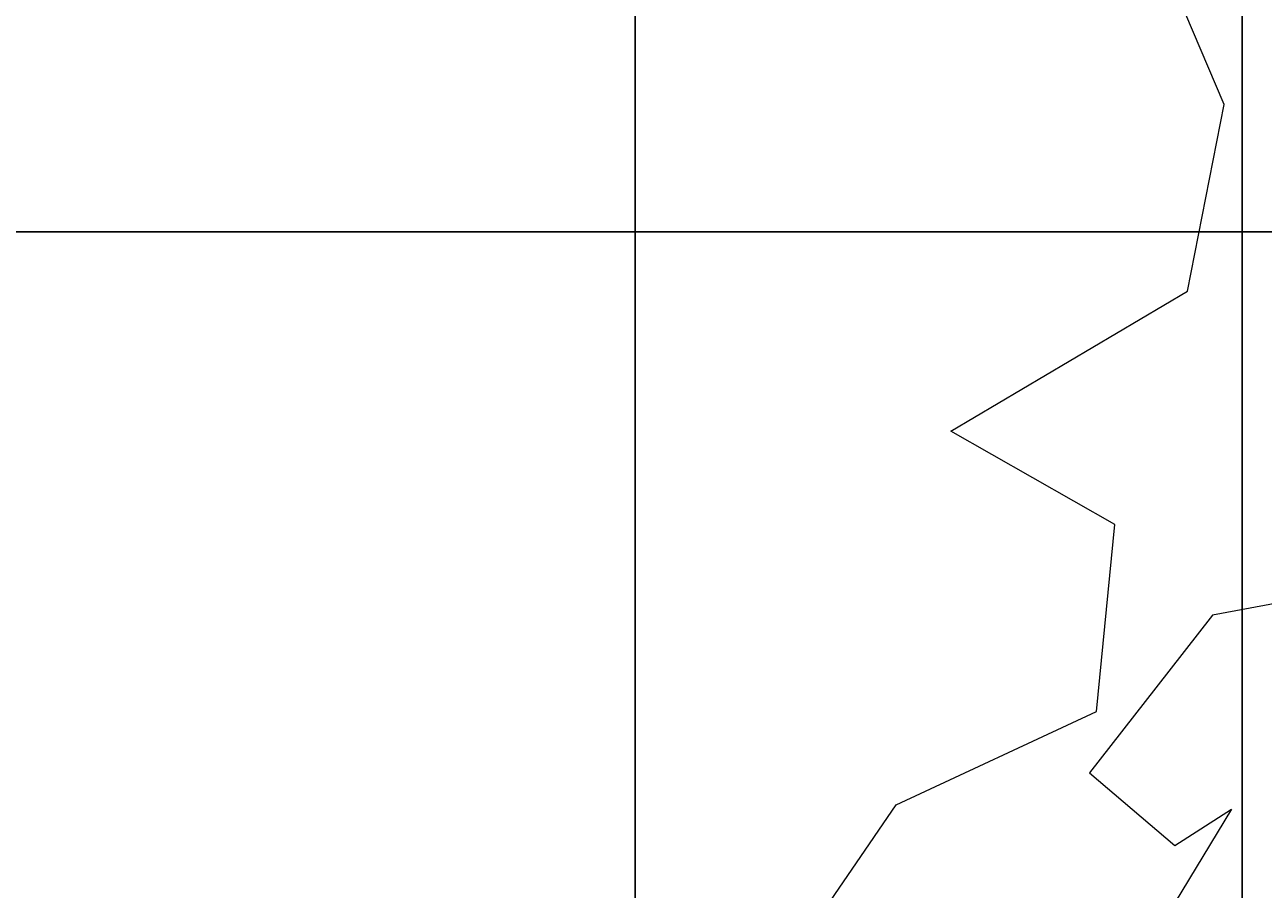
# Model space of a CAD drawing. Units: inches. Extents: x -26 to 776, y -22 to 650.
# Tile 48 of 62: x 506 to 586, y 102 to 158. Entities that reach past the tile are written whole.
import ezdxf

# ---------------------------------------------------------------- set-up
doc = ezdxf.new("R2010")
doc.units = ezdxf.units.IN
doc.header["$MEASUREMENT"] = 0
doc.layers.add('A-ANNO-DIMS', color=2, linetype='Continuous', lineweight=18)
doc.layers.add('L-PLNT-TREE', color=94, linetype='Continuous', lineweight=18)
doc.styles.get("Standard").update_dxf_attribs({"font": 'arial.ttf'})
doc.dimstyles.get("Standard").update_dxf_attribs({"dimtxt": 0.5625, "dimasz": 0.18, "dimexe": 0.18, "dimexo": 0.0625, "dimgap": 0.09, "dimtad": 0, "dimtih": 1, "dimtoh": 1, "dimdec": 4, "dimzin": 0, "dimdsep": 46, "dimlunit": 4, "dimtxsty": 'Standard', "dimcen": 0.09, "dimadec": 0, "dimazin": 0, "dimtfac": 1, "dimtdec": 4, "dimtofl": 0, "dimtmove": 0, "dimatfit": 3, "dimfxl": 1, "dimtolj": 1, "dimtzin": 0, "dimarcsym": 0})

# ---------------------------------------------------------------- blocks, each defined once
blk = doc.blocks.new('Tree - type 3 evergreen elevation')
blk.add_lwpolyline([(-39.2518, 74.099), (-42.2711, 73.5461), (-44.8592, 70.2282), (-47.8786, 66.3574), (-43.9965, 63.0395), (-41.4085, 64.6985), (-44.3346, 59.8898)])
blk = doc.blocks.new('Tree - type 2 deciduous elevation')
blk.add_lwpolyline([(19.675, 39.077), (23.701, 44.975), (30.027, 47.924), (30.602, 53.823), (25.426, 56.772), (32.903, 61.196), (34.053, 67.094), (30.602, 75.205), (34.628, 89.951), (26.576, 103.222)])
blk = doc.blocks.new('*D20')
at = {"layer": 'A-ANNO-DIMS', "color": 0, "lineweight": -2, "transparency": 16777216}
for p, q in [((425.806, 455.472), (775.335, 455.472)), ((775.155, 455.292), (775.155, 235.854)), ((775.155, 15.662), (775.155, 235.1)), ((425.806, 15.482), (775.335, 15.482))]:
    blk.add_line(p, q, dxfattribs=at)
at = {"layer": 'A-ANNO-DIMS', "color": 0, "transparency": 16777216}
for points in [[(775.125, 455.292), (775.185, 455.292), (775.155, 455.472)], [(775.125, 15.662), (775.185, 15.662), (775.155, 15.482)]]:
    blk.add_solid(points, dxfattribs=at)
at = {"layer": 'Defpoints', "color": 0, "transparency": 16777216}
for p in [(425.743, 455.472), (775.155, 455.472), (425.743, 15.482)]:
    blk.add_point(p, dxfattribs=at)
at = {"layer": 'A-ANNO-DIMS', "color": 0, "transparency": 16777216, "insert": (775.155, 235.477), "char_height": 0.5625, "attachment_point": 5}
blk.add_mtext('\\A1;440', dxfattribs=at)
blk = doc.blocks.new('*D30')
at = {"layer": 'A-ANNO-DIMS', "color": 0, "lineweight": -2, "transparency": 16777216}
for p, q in [((280.68, 144.836), (775.335, 144.836)), ((775.155, 144.656), (775.155, 86.007)), ((775.155, 26.604), (775.155, 85.253)), ((280.68, 26.424), (775.335, 26.424))]:
    blk.add_line(p, q, dxfattribs=at)
at = {"layer": 'A-ANNO-DIMS', "color": 0, "transparency": 16777216}
for points in [[(775.125, 144.656), (775.185, 144.656), (775.155, 144.836)], [(775.125, 26.604), (775.185, 26.604), (775.155, 26.424)]]:
    blk.add_solid(points, dxfattribs=at)
at = {"layer": 'Defpoints', "color": 0, "transparency": 16777216}
for p in [(280.617, 144.836), (775.155, 144.836), (280.617, 26.424)]:
    blk.add_point(p, dxfattribs=at)
at = {"layer": 'A-ANNO-DIMS', "color": 0, "transparency": 16777216, "insert": (775.155, 85.63), "char_height": 0.5625, "attachment_point": 5}
blk.add_mtext('\\A1;118.41', dxfattribs=at)
blk = doc.blocks.new('*D45')
at = {"layer": 'A-ANNO-DIMS', "color": 0, "lineweight": -2, "transparency": 16777216}
for p, q in [((507.738, 408.639), (775.335, 408.639)), ((775.155, 408.459), (775.155, 212.438)), ((775.155, 15.662), (775.155, 211.683)), ((585.998, 15.482), (775.335, 15.482))]:
    blk.add_line(p, q, dxfattribs=at)
at = {"layer": 'A-ANNO-DIMS', "color": 0, "transparency": 16777216}
for points in [[(775.125, 408.459), (775.185, 408.459), (775.155, 408.639)], [(775.125, 15.662), (775.185, 15.662), (775.155, 15.482)]]:
    blk.add_solid(points, dxfattribs=at)
at = {"layer": 'Defpoints', "color": 0, "transparency": 16777216}
for p in [(507.676, 408.639), (775.155, 408.639), (585.935, 15.482)]:
    blk.add_point(p, dxfattribs=at)
at = {"layer": 'A-ANNO-DIMS', "color": 0, "transparency": 16777216, "insert": (775.155, 212.061), "char_height": 0.5625, "attachment_point": 5}
blk.add_mtext('\\A1;393.16', dxfattribs=at)
blk = doc.blocks.new('*D47')
at = {"layer": 'A-ANNO-DIMS', "color": 0, "lineweight": -2, "transparency": 16777216}
for p, q in [((584.343, 199.901), (584.343, -21.315)), ((428.648, 180.243), (428.648, -21.315)), ((428.828, -21.135), (505.483, -21.135)), ((584.163, -21.135), (507.508, -21.135))]:
    blk.add_line(p, q, dxfattribs=at)
at = {"layer": 'A-ANNO-DIMS', "color": 0, "transparency": 16777216}
for points in [[(428.828, -21.105), (428.828, -21.165), (428.648, -21.135)], [(584.163, -21.105), (584.163, -21.165), (584.343, -21.135)]]:
    blk.add_solid(points, dxfattribs=at)
at = {"layer": 'Defpoints', "color": 0, "transparency": 16777216}
for p in [(584.343, 199.963), (428.648, 180.305), (584.343, -21.135)]:
    blk.add_point(p, dxfattribs=at)
at = {"layer": 'A-ANNO-DIMS', "color": 0, "transparency": 16777216, "insert": (506.496, -21.135), "char_height": 0.5625, "attachment_point": 5}
blk.add_mtext('\\A1;155.7', dxfattribs=at)
blk = doc.blocks.new('*D48')
at = {"layer": 'A-ANNO-DIMS', "color": 0, "lineweight": -2, "transparency": 16777216}
for p, q in [((545.033, 67.415), (545.033, 649.856)), ((545.213, 649.676), (640.879, 649.676)), ((738.57, 649.676), (642.904, 649.676)), ((738.75, 50.911), (738.75, 649.856))]:
    blk.add_line(p, q, dxfattribs=at)
at = {"layer": 'A-ANNO-DIMS', "color": 0, "transparency": 16777216}
for points in [[(545.213, 649.706), (545.213, 649.646), (545.033, 649.676)], [(738.57, 649.706), (738.57, 649.646), (738.75, 649.676)]]:
    blk.add_solid(points, dxfattribs=at)
at = {"layer": 'Defpoints', "color": 0, "transparency": 16777216}
for p in [(738.75, 649.676), (545.033, 67.352), (738.75, 50.848)]:
    blk.add_point(p, dxfattribs=at)
at = {"layer": 'A-ANNO-DIMS', "color": 0, "transparency": 16777216, "insert": (641.892, 649.676), "char_height": 0.5625, "attachment_point": 5}
blk.add_mtext('\\A1;193.7', dxfattribs=at)

msp = doc.modelspace()

# ---------------------------------------------------------------- block references
at = {"layer": 'L-PLNT-TREE'}
for name, p, xscale, yscale, zscale in [('Tree - type 2 deciduous elevation', (513.3241, 15.4824), 2.050905272406618, 2.050905272406618, 2.050905272406618), ('Tree - type 3 evergreen elevation', (642.5048, 15.4824), 1.421226385586178, 1.421226385586178, 1.421226385586178)]:
    msp.add_blockref(name, p, dxfattribs=dict(at, xscale=xscale, yscale=yscale, zscale=zscale))

# ---------------------------------------------------------------- dimensions: what is measured, and where the dimension line sits
at = {"layer": 'A-ANNO-DIMS'}
for base, p1, p2, picture, middle in [((738.7503, 649.6763), (545.0331, 67.3523), (738.7503, 50.8482), '*D48', (641.8917, 649.6763)), ((584.3428, -21.1349), (428.6484, 180.3054), (584.3428, 199.9634), '*D47', (506.4956, -21.1349))]:
    dim = msp.add_linear_dim(base=base, p1=p1, p2=p2, dimstyle='Standard', override={"dimdec": 1, "dimlfac": 1, "dimrnd": 0, "dimzin": 0, "dimdsep": 46, "dimlunit": 2}, dxfattribs=at)
    dim.commit()
    dim.dimension.update_dxf_attribs({"geometry": picture, "text_midpoint": middle})
for base, p1, p2, override, picture, middle in [((775.1553, 455.4717), (425.7434, 15.4824), (425.7434, 455.4717), {"dimdec": 0, "dimlfac": 1, "dimrnd": 0, "dimzin": 0, "dimdsep": 46, "dimlunit": 2}, '*D20', (775.1553, 235.477)), ((775.1553, 408.6389), (585.9354, 15.4824), (507.6759, 408.6389), {"dimdec": 2, "dimlfac": 1, "dimrnd": 0, "dimzin": 0, "dimdsep": 46, "dimlunit": 2}, '*D45', (775.1553, 212.0606)), ((775.1553, 144.8359), (280.6173, 26.4239), (280.6173, 144.8359), {"dimdec": 2, "dimlfac": 1, "dimrnd": 0, "dimzin": 0, "dimdsep": 46, "dimlunit": 2}, '*D30', (775.1553, 85.6299))]:
    dim = msp.add_linear_dim(base=base, p1=p1, p2=p2, angle=90, dimstyle='Standard', override=override, dxfattribs=at)
    dim.commit()
    dim.dimension.update_dxf_attribs({"geometry": picture, "text_midpoint": middle})

doc.saveas('drawing.dxf')
